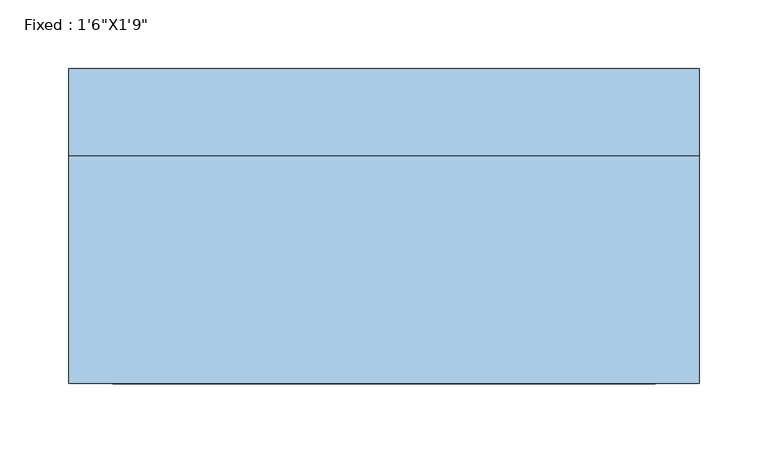
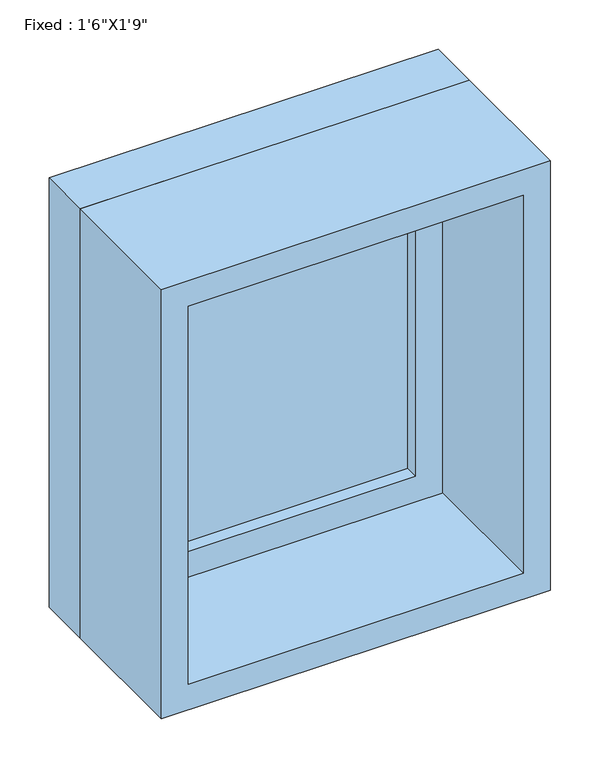
"""IFC4 building model written with IfcOpenShell, lengths in millimetres: window geometry."""

from ifc_helpers import new_model, si_unit, frame, origin, place, context, project, spatial, polyline, outline, extrude, source, transform, mapped, element, save


def window_abb441dd(model_context):
    return source(origin(), model_context, "Body", "SweptSolid", [
        extrude(outline(polyline([(127.0, 66.675), (-203.2, 66.675), (-203.2, 79.375), (127.0, 79.375), (127.0, 66.675)])), frame((0.0, 0.0, 2197.1), z_axis=(0.0, 0.0, 1.0), x_axis=(1.0, 0.0, 0.0)), (0.0, 0.0, 1.0), 406.4),
        extrude(outline(polyline([(2647.95, -247.65), (2152.65, -247.65), (2152.65, 171.45), (2647.95, 171.45), (2647.95, -247.65)]), holes=[polyline([(2603.5, -203.2), (2603.5, 127.0), (2197.1, 127.0), (2197.1, -203.2), (2603.5, -203.2)])]), frame((0.0, 50.8, 0.0), z_axis=(0.0, 1.0, 0.0), x_axis=(0.0, 0.0, 1.0)), (0.0, 0.0, 1.0), 44.45),
        extrude(outline(polyline([(2667.0, -266.7), (2133.6, -266.7), (2133.6, 190.5), (2667.0, 190.5), (2667.0, -266.7)]), holes=[polyline([(2635.25, -234.95), (2635.25, 158.75), (2165.35, 158.75), (2165.35, -234.95), (2635.25, -234.95)])]), frame((0.0, -114.3, 0.0), z_axis=(0.0, 1.0, 0.0), x_axis=(0.0, 0.0, 1.0)), (0.0, 0.0, 1.0), 165.1),
        extrude(outline(polyline([(2667.0, 190.5), (2667.0, -266.7), (2133.6, -266.7), (2133.6, 190.5), (2667.0, 190.5)]), holes=[polyline([(2647.95, 171.45), (2152.65, 171.45), (2152.65, -247.65), (2647.95, -247.65), (2647.95, 171.45)])]), frame((0.0, 50.8, 0.0), z_axis=(0.0, 1.0, 0.0), x_axis=(0.0, 0.0, 1.0)), (0.0, 0.0, 1.0), 63.5),
    ])


if __name__ == "__main__":
    model = new_model("IFC4")
    model_context = context("Model", 3, world=origin())
    ifc_project = project(units=[si_unit("LENGTHUNIT", "METRE", prefix="MILLI")], contexts=[model_context])
    site = spatial("IfcSite", under=ifc_project)
    building = spatial("IfcBuilding", under=site)
    placement = place(None, origin())
    window_shape = window_abb441dd(model_context)
    element("IfcWindow", 1, ObjectType="Fixed : 1'6\"X1'9\"", at=placement, inside=building, context=model_context, shape_type="MappedRepresentation", body=[
        mapped(window_shape, transform((0.0, 0.0, 0.0), x_axis=(1.0, 0.0, 0.0), y_axis=(0.0, 1.0, 0.0), z_axis=(0.0, 0.0, 1.0))),
    ])
    save(model, "model.ifc")

# Revit data of these elements
# Type "Fixed : 1'6\"X1'9\""
#   Type Mark = "24"
#   Construction Type Id = "GSP4R"
#   Assembly Code = "B2020100"
#   Analytic Construction = "1/8 in Pilkington single glazing"
#   Visual Light Transmittance = 0.9
#   Solar Heat Gain Coefficient = 0.78
#   Heat Transfer Coefficient (U) = 0.6496 BTU/(h·ft²·°F)
#   Height = 1' - 9"
#   Default Sill Height = 7' - 0"
#   Width = 1' - 6"
#   Window Inset = 0' - 0 3/4"
#   Define Thermal Properties by = 1
#   Glass Pane Material = Glass
#   Sash Material = Sash
#   Wall Closure = (empty or 0)
# Element 1 (IfcWindow, "Fixed : 1'6\"X1'9\"")
#   Materials on its faces: "Sash", "Glass"
# Materials
#   "Glass": class "Glass", colour RGB 0 128 192, transparency 0.75, Description = "Soda Lime Glass", Cost = 0
#   "Sash": class "Wood", colour RGB 224 178 126, transparency 0, Cost = 0
